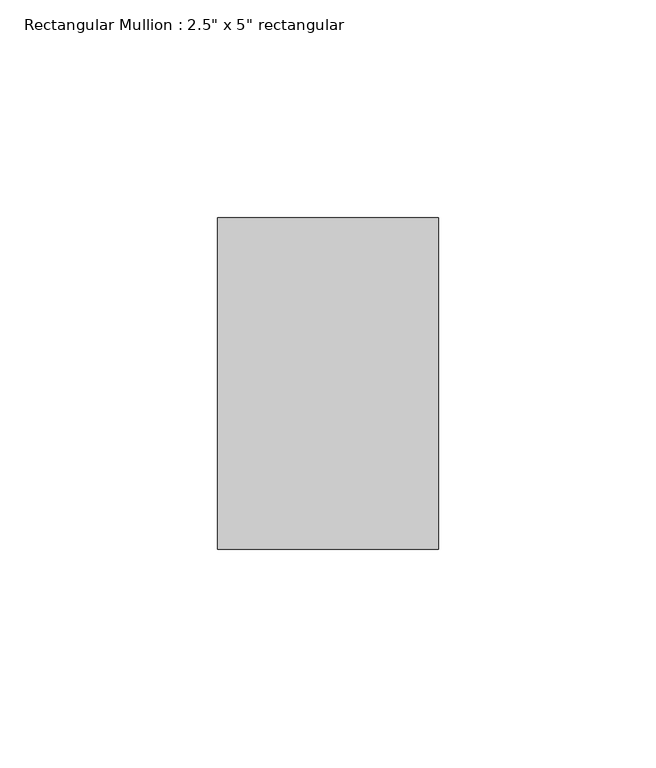
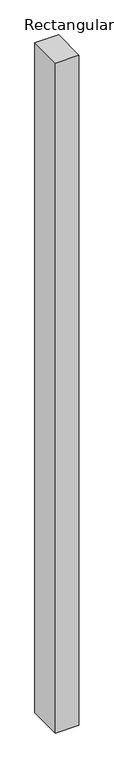
"""IFC4 building model written with IfcOpenShell, lengths in millimetres: member geometry."""

from ifc_helpers import new_model, si_unit, frame, origin, place, context, project, spatial, polyline, outline, extrude, source, transform, mapped, element, save


def member_19d0c1c6(model_context):
    return source(origin(), model_context, "Body", "SweptSolid", [
        extrude(outline(polyline([(0.0, 38.1), (0.0, -38.1), (-50.8, -38.1), (-50.8, 38.1), (0.0, 38.1)])), frame((0.0, 0.0, -1524.0), z_axis=(0.0, 0.0, 1.0), x_axis=(1.0, 0.0, 0.0)), (0.0, 0.0, 1.0), 1524.0),
    ])


if __name__ == "__main__":
    model = new_model("IFC4")
    model_context = context("Model", 3, world=origin())
    ifc_project = project(units=[si_unit("LENGTHUNIT", "METRE", prefix="MILLI")], contexts=[model_context])
    site = spatial("IfcSite", under=ifc_project)
    building = spatial("IfcBuilding", under=site)
    placement = place(None, origin())
    member_shape = member_19d0c1c6(model_context)
    element("IfcMember", 1, ObjectType="Rectangular Mullion : 2.5\" x 5\" rectangular", at=placement, inside=building, context=model_context, shape_type="MappedRepresentation", body=[
        mapped(member_shape, transform((0.0, 0.0, 0.0), x_axis=(1.0, 0.0, 0.0), y_axis=(0.0, 1.0, 0.0), z_axis=(0.0, 0.0, 1.0))),
    ])
    save(model, "model.ifc")

# Revit data of these elements
# Type "Rectangular Mullion : 2.5\" x 5\" rectangular"
#   built-in parameter 1007304 = 0.25 (stored number, unit not read)
#   built-in parameter 1007301 = 0.0833333 (stored number, unit not read)
#   built-in parameter 1007300 = 0.0833333 (stored number, unit not read)
# Element 1 (IfcMember, "Rectangular Mullion : 2.5\" x 5\" rectangular")
#   Materials on its faces: "Aluminum"
# Materials
#   "Aluminum": class "Metal", colour RGB 244 245 246, transparency 0, Description = "Aluminum 6061", Cost = 0
